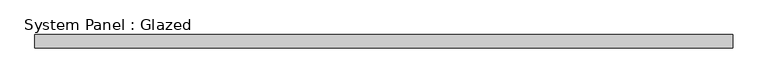
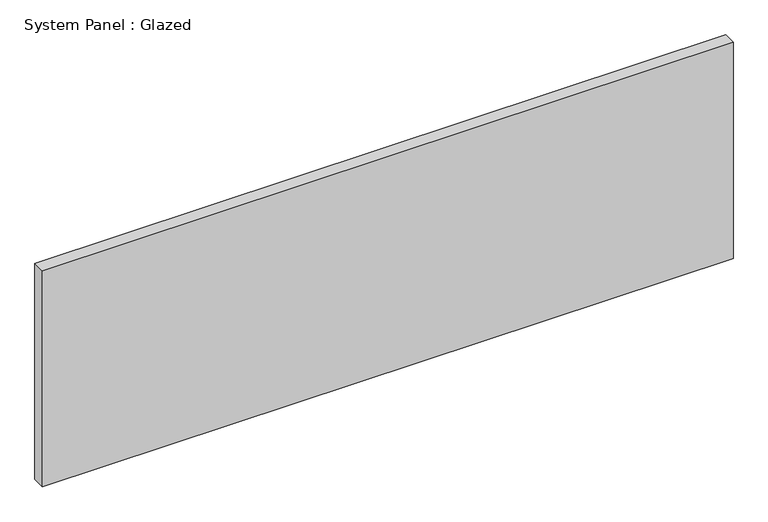
"""IFC4 building model written with IfcOpenShell, lengths in millimetres: plate geometry, System Panel : Glazed."""

from ifc_helpers import new_model, si_unit, origin, origin_with_axes, place, context, project, spatial, polyline, outline, extrude, source, transform, mapped, element, save


def system_panel_glazed_b8f86fea(model_context):
    return source(origin(), model_context, "Body", "SweptSolid", [
        extrude(outline(polyline([(670.9833332, 19.05), (-670.9833332, 19.05), (-670.9833332, 44.45), (670.9833332, 44.45), (670.9833332, 19.05)])), origin_with_axes(), (0.0, 0.0, 1.0), 444.5),
    ])


if __name__ == "__main__":
    model = new_model("IFC4")
    model_context = context("Model", 3, world=origin())
    ifc_project = project(units=[si_unit("LENGTHUNIT", "METRE", prefix="MILLI")], contexts=[model_context])
    site = spatial("IfcSite", under=ifc_project)
    building = spatial("IfcBuilding", under=site)
    placement = place(None, origin())
    system_panel_glazed_shape = system_panel_glazed_b8f86fea(model_context)
    element("IfcPlate", 1, ObjectType="System Panel : Glazed", at=placement, inside=building, context=model_context, shape_type="MappedRepresentation", body=[
        mapped(system_panel_glazed_shape, transform((0.0, 0.0, 0.0), x_axis=(1.0, 0.0, 0.0), y_axis=(0.0, 1.0, 0.0), z_axis=(0.0, 0.0, 1.0))),
    ])
    save(model, "model.ifc")

# Revit data of these elements
# Type "System Panel : Glazed"
#   Construction Type Id = "GSP4R"
#   Analytic Construction = "1/8 in Pilkington single glazing"
#   Visual Light Transmittance = 0.9
#   Solar Heat Gain Coefficient = 0.86
#   Heat Transfer Coefficient (U) = 1.18115 BTU/(h·ft²·°F)
#   Define Thermal Properties by = 1
# Element 1 (IfcPlate, "System Panel : Glazed")
#   Materials on its faces: "glass panel 223"
# Materials
#   "glass panel 223": class "Generic", colour RGB 120 120 120, transparency 0, Cost = 0
